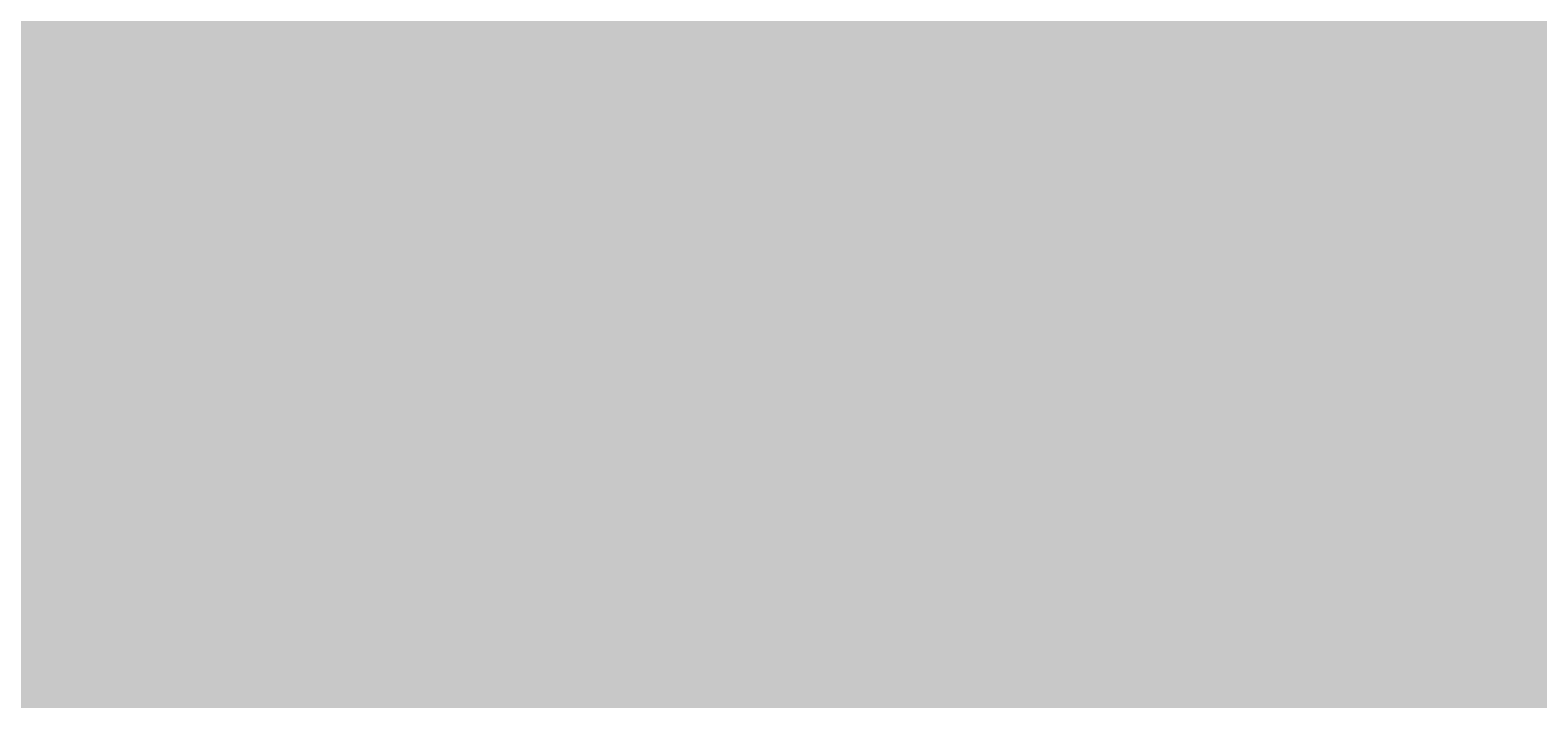
# Model space of a CAD drawing. Units: millimetres. Extents: x -22994 to 29398, y -19990 to 20176.
# Tile 108 of 135: x 237 to 296, y 98 to 124. Entities that reach past the tile are written whole.
import ezdxf

# ---------------------------------------------------------------- set-up
doc = ezdxf.new("R2010")
doc.units = ezdxf.units.MM
doc.header["$MEASUREMENT"] = 0
doc.layers.add('M-DIMS', color=2, linetype='Continuous', lineweight=18)
doc.styles.get("Standard").update_dxf_attribs({"font": 'arial.ttf'})
doc.dimstyles.get("Standard").update_dxf_attribs({"dimtxt": 0.18, "dimasz": 10000, "dimexe": 0.18, "dimexo": 0.0625, "dimgap": 0.09, "dimtad": 0, "dimtih": 1, "dimtoh": 1, "dimdec": 0, "dimzin": 0, "dimdsep": 46, "dimtxsty": 'Standard', "dimcen": 0.09, "dimadec": 0, "dimazin": 0, "dimtfac": 1, "dimtdec": 0, "dimtofl": 0, "dimtmove": 0, "dimatfit": 3, "dimfxl": 1, "dimtolj": 1, "dimtzin": 0, "dimlwd": 30, "dimarcsym": 0})

# ---------------------------------------------------------------- blocks, each defined once
blk = doc.blocks.new('*D2')
at = {"layer": 'Defpoints', "color": 0, "transparency": 16777216}
for p in [(6.677, 10.271), (290.852, 10.271), (290.852, -5.079)]:
    blk.add_point(p, dxfattribs=at)
at = {"layer": 'M-DIMS', "color": 0, "lineweight": -2, "transparency": 16777216}
for p, q in [((6.677, 10.209), (6.677, -5.259)), ((290.852, 10.209), (290.852, -5.259))]:
    blk.add_line(p, q, dxfattribs=at)
at = {"layer": 'M-DIMS', "color": 0, "lineweight": 30, "transparency": 16777216}
for p, q in [((-9993.323, -5.079), (-19993.323, -5.079)), ((10290.852, -5.079), (20290.852, -5.079))]:
    blk.add_line(p, q, dxfattribs=at)
at = {"layer": 'M-DIMS', "color": 0, "transparency": 16777216}
for points in [[(-9993.323, 1661.588), (-9993.323, -1671.745), (6.677, -5.079)], [(10290.852, 1661.588), (10290.852, -1671.745), (290.852, -5.079)]]:
    blk.add_solid(points, dxfattribs=at)
at = {"layer": 'M-DIMS', "color": 0, "transparency": 16777216, "insert": (148.765, -5.079), "char_height": 0.18, "attachment_point": 5}
blk.add_mtext('\\A1;284.2', dxfattribs=at)
blk = doc.blocks.new('*D3')
at = {"layer": 'Defpoints', "color": 0, "transparency": 16777216}
for p in [(110.265, 204.165), (110.265, 176.366), (95.833, 127.967)]:
    blk.add_point(p, dxfattribs=at)
at = {"layer": 'M-DIMS', "color": 0, "lineweight": -2, "transparency": 16777216}
for p, q in [((95.833, 128.03), (95.833, 204.345)), ((110.265, 176.429), (110.265, 204.345))]:
    blk.add_line(p, q, dxfattribs=at)
at = {"layer": 'M-DIMS', "color": 0, "lineweight": 30, "transparency": 16777216}
for p, q in [((-9904.167, 204.165), (-19904.167, 204.165)), ((10110.265, 204.165), (20110.265, 204.165))]:
    blk.add_line(p, q, dxfattribs=at)
at = {"layer": 'M-DIMS', "color": 0, "transparency": 16777216}
for points in [[(-9904.167, 1870.832), (-9904.167, -1462.501), (95.833, 204.165)], [(10110.265, 1870.832), (10110.265, -1462.501), (110.265, 204.165)]]:
    blk.add_solid(points, dxfattribs=at)
at = {"layer": 'M-DIMS', "color": 0, "transparency": 16777216, "insert": (103.049, 204.165), "char_height": 0.18, "attachment_point": 5}
blk.add_mtext('\\A1;14.432', dxfattribs=at)
blk = doc.blocks.new('*D4')
at = {"layer": 'Defpoints', "color": 0, "transparency": 16777216}
for p in [(116.265, 204.165), (110.265, 176.366), (116.265, 176.366)]:
    blk.add_point(p, dxfattribs=at)
at = {"layer": 'M-DIMS', "color": 0, "lineweight": -2, "transparency": 16777216}
for p, q in [((110.265, 176.429), (110.265, 204.345)), ((116.265, 176.429), (116.265, 204.345))]:
    blk.add_line(p, q, dxfattribs=at)
at = {"layer": 'M-DIMS', "color": 0, "lineweight": 30, "transparency": 16777216}
for p, q in [((-9889.735, 204.165), (-19889.735, 204.165)), ((10116.265, 204.165), (20116.265, 204.165))]:
    blk.add_line(p, q, dxfattribs=at)
at = {"layer": 'M-DIMS', "color": 0, "transparency": 16777216}
for points in [[(-9889.735, 1870.832), (-9889.735, -1462.501), (110.265, 204.165)], [(10116.265, 1870.832), (10116.265, -1462.501), (116.265, 204.165)]]:
    blk.add_solid(points, dxfattribs=at)
at = {"layer": 'M-DIMS', "color": 0, "transparency": 16777216, "insert": (113.265, 204.165), "char_height": 0.18, "attachment_point": 5}
blk.add_mtext('\\A1;6', dxfattribs=at)
blk = doc.blocks.new('*D5')
at = {"layer": 'Defpoints', "color": 0, "transparency": 16777216}
for p in [(181.265, 204.165), (116.265, 176.366), (181.265, 176.366)]:
    blk.add_point(p, dxfattribs=at)
at = {"layer": 'M-DIMS', "color": 0, "lineweight": -2, "transparency": 16777216}
for p, q in [((116.265, 176.429), (116.265, 204.345)), ((181.265, 176.429), (181.265, 204.345))]:
    blk.add_line(p, q, dxfattribs=at)
at = {"layer": 'M-DIMS', "color": 0, "lineweight": 30, "transparency": 16777216}
for p, q in [((-9883.735, 204.165), (-19883.735, 204.165)), ((10181.265, 204.165), (20181.265, 204.165))]:
    blk.add_line(p, q, dxfattribs=at)
at = {"layer": 'M-DIMS', "color": 0, "transparency": 16777216}
for points in [[(-9883.735, 1870.832), (-9883.735, -1462.501), (116.265, 204.165)], [(10181.265, 1870.832), (10181.265, -1462.501), (181.265, 204.165)]]:
    blk.add_solid(points, dxfattribs=at)
at = {"layer": 'M-DIMS', "color": 0, "transparency": 16777216, "insert": (148.765, 204.165), "char_height": 0.18, "attachment_point": 5}
blk.add_mtext('\\A1;65', dxfattribs=at)
blk = doc.blocks.new('*D6')
at = {"layer": 'Defpoints', "color": 0, "transparency": 16777216}
for p in [(187.265, 204.165), (181.265, 176.366), (187.265, 176.366)]:
    blk.add_point(p, dxfattribs=at)
at = {"layer": 'M-DIMS', "color": 0, "lineweight": -2, "transparency": 16777216}
for p, q in [((181.265, 176.429), (181.265, 204.345)), ((187.265, 176.429), (187.265, 204.345))]:
    blk.add_line(p, q, dxfattribs=at)
at = {"layer": 'M-DIMS', "color": 0, "lineweight": 30, "transparency": 16777216}
for p, q in [((-9818.735, 204.165), (-19818.735, 204.165)), ((10187.265, 204.165), (20187.265, 204.165))]:
    blk.add_line(p, q, dxfattribs=at)
at = {"layer": 'M-DIMS', "color": 0, "transparency": 16777216}
for points in [[(-9818.735, 1870.832), (-9818.735, -1462.501), (181.265, 204.165)], [(10187.265, 1870.832), (10187.265, -1462.501), (187.265, 204.165)]]:
    blk.add_solid(points, dxfattribs=at)
at = {"layer": 'M-DIMS', "color": 0, "transparency": 16777216, "insert": (184.265, 204.165), "char_height": 0.18, "attachment_point": 5}
blk.add_mtext('\\A1;6', dxfattribs=at)
blk = doc.blocks.new('*D7')
at = {"layer": 'Defpoints', "color": 0, "transparency": 16777216}
for p in [(201.697, 204.165), (187.265, 176.366), (201.697, 127.967)]:
    blk.add_point(p, dxfattribs=at)
at = {"layer": 'M-DIMS', "color": 0, "lineweight": -2, "transparency": 16777216}
for p, q in [((187.265, 176.429), (187.265, 204.345)), ((201.697, 128.03), (201.697, 204.345))]:
    blk.add_line(p, q, dxfattribs=at)
at = {"layer": 'M-DIMS', "color": 0, "lineweight": 30, "transparency": 16777216}
for p, q in [((-9812.735, 204.165), (-19812.735, 204.165)), ((10201.697, 204.165), (20201.697, 204.165))]:
    blk.add_line(p, q, dxfattribs=at)
at = {"layer": 'M-DIMS', "color": 0, "transparency": 16777216}
for points in [[(-9812.735, 1870.832), (-9812.735, -1462.501), (187.265, 204.165)], [(10201.697, 1870.832), (10201.697, -1462.501), (201.697, 204.165)]]:
    blk.add_solid(points, dxfattribs=at)
at = {"layer": 'M-DIMS', "color": 0, "transparency": 16777216, "insert": (194.481, 204.165), "char_height": 0.18, "attachment_point": 5}
blk.add_mtext('\\A1;14.432', dxfattribs=at)
blk = doc.blocks.new('*D8')
at = {"layer": 'Defpoints', "color": 0, "transparency": 16777216}
for p in [(227.648, 204.165), (227.648, 146.73), (201.697, 127.967)]:
    blk.add_point(p, dxfattribs=at)
at = {"layer": 'M-DIMS', "color": 0, "lineweight": -2, "transparency": 16777216}
for p, q in [((201.697, 128.03), (201.697, 204.345)), ((227.648, 146.792), (227.648, 204.345))]:
    blk.add_line(p, q, dxfattribs=at)
at = {"layer": 'M-DIMS', "color": 0, "lineweight": 30, "transparency": 16777216}
for p, q in [((-9798.303, 204.165), (-19798.303, 204.165)), ((10227.648, 204.165), (20227.648, 204.165))]:
    blk.add_line(p, q, dxfattribs=at)
at = {"layer": 'M-DIMS', "color": 0, "transparency": 16777216}
for points in [[(-9798.303, 1870.832), (-9798.303, -1462.501), (201.697, 204.165)], [(10227.648, 1870.832), (10227.648, -1462.501), (227.648, 204.165)]]:
    blk.add_solid(points, dxfattribs=at)
at = {"layer": 'M-DIMS', "color": 0, "transparency": 16777216, "insert": (214.673, 204.165), "char_height": 0.18, "attachment_point": 5}
blk.add_mtext('\\A1;25.95', dxfattribs=at)
blk = doc.blocks.new('*D9')
at = {"layer": 'Defpoints', "color": 0, "transparency": 16777216}
for p in [(187.265, 176.366), (306.202, 176.366), (290.852, 10.271)]:
    blk.add_point(p, dxfattribs=at)
at = {"layer": 'M-DIMS', "color": 0, "lineweight": 30, "transparency": 16777216}
for p, q in [((306.202, 10176.366), (306.202, 20176.366)), ((306.202, -9989.729), (306.202, -19989.729))]:
    blk.add_line(p, q, dxfattribs=at)
at = {"layer": 'M-DIMS', "color": 0, "lineweight": -2, "transparency": 16777216}
for p, q in [((187.327, 176.366), (306.382, 176.366)), ((290.915, 10.271), (306.382, 10.271))]:
    blk.add_line(p, q, dxfattribs=at)
at = {"layer": 'M-DIMS', "color": 0, "transparency": 16777216}
for points in [[(-1360.465, 10176.366), (1972.869, 10176.366), (306.202, 176.366)], [(-1360.465, -9989.729), (1972.869, -9989.729), (306.202, 10.271)]]:
    blk.add_solid(points, dxfattribs=at)
at = {"layer": 'M-DIMS', "color": 0, "transparency": 16777216, "insert": (306.202, 93.319), "char_height": 0.18, "attachment_point": 5}
blk.add_mtext('\\A1;166.1', dxfattribs=at)
blk = doc.blocks.new('*D10')
at = {"layer": 'Defpoints', "color": 0, "transparency": 16777216}
for p in [(125.65, 136.071), (133.346, 136.071), (133.346, -5.079)]:
    blk.add_point(p, dxfattribs=at)
at = {"layer": 'M-DIMS', "color": 0, "lineweight": -2, "transparency": 16777216}
for p, q in [((125.65, 136.009), (125.65, -5.259)), ((133.346, 136.009), (133.346, -5.259))]:
    blk.add_line(p, q, dxfattribs=at)
at = {"layer": 'M-DIMS', "color": 0, "lineweight": 30, "transparency": 16777216}
for p, q in [((-9874.35, -5.079), (-19874.35, -5.079)), ((10133.346, -5.079), (20133.346, -5.079))]:
    blk.add_line(p, q, dxfattribs=at)
at = {"layer": 'M-DIMS', "color": 0, "transparency": 16777216}
for points in [[(-9874.35, 1661.588), (-9874.35, -1671.745), (125.65, -5.079)], [(10133.346, 1661.588), (10133.346, -1671.745), (133.346, -5.079)]]:
    blk.add_solid(points, dxfattribs=at)
at = {"layer": 'M-DIMS', "color": 0, "transparency": 16777216, "insert": (129.498, -5.079), "char_height": 0.18, "attachment_point": 5}
blk.add_mtext('\\A1;7.696', dxfattribs=at)
blk = doc.blocks.new('*D11')
at = {"layer": 'Defpoints', "color": 0, "transparency": 16777216}
for p in [(133.346, 136.071), (135.65, 136.071), (135.65, -5.079)]:
    blk.add_point(p, dxfattribs=at)
at = {"layer": 'M-DIMS', "color": 0, "lineweight": -2, "transparency": 16777216}
for p, q in [((133.346, 136.009), (133.346, -5.259)), ((135.65, 136.009), (135.65, -5.259))]:
    blk.add_line(p, q, dxfattribs=at)
at = {"layer": 'M-DIMS', "color": 0, "lineweight": 30, "transparency": 16777216}
for p, q in [((-9866.654, -5.079), (-19866.654, -5.079)), ((10135.65, -5.079), (20135.65, -5.079))]:
    blk.add_line(p, q, dxfattribs=at)
at = {"layer": 'M-DIMS', "color": 0, "transparency": 16777216}
for points in [[(-9866.654, 1661.588), (-9866.654, -1671.745), (133.346, -5.079)], [(10135.65, 1661.588), (10135.65, -1671.745), (135.65, -5.079)]]:
    blk.add_solid(points, dxfattribs=at)
at = {"layer": 'M-DIMS', "color": 0, "transparency": 16777216, "insert": (134.498, -5.079), "char_height": 0.18, "attachment_point": 5}
blk.add_mtext('\\A1;2.304', dxfattribs=at)
blk = doc.blocks.new('*D12')
at = {"layer": 'Defpoints', "color": 0, "transparency": 16777216}
for p in [(135.65, 136.071), (145.65, 136.071), (145.65, -5.079)]:
    blk.add_point(p, dxfattribs=at)
at = {"layer": 'M-DIMS', "color": 0, "lineweight": -2, "transparency": 16777216}
for p, q in [((135.65, 136.009), (135.65, -5.259)), ((145.65, 136.009), (145.65, -5.259))]:
    blk.add_line(p, q, dxfattribs=at)
at = {"layer": 'M-DIMS', "color": 0, "lineweight": 30, "transparency": 16777216}
for p, q in [((-9864.35, -5.079), (-19864.35, -5.079)), ((10145.65, -5.079), (20145.65, -5.079))]:
    blk.add_line(p, q, dxfattribs=at)
at = {"layer": 'M-DIMS', "color": 0, "transparency": 16777216}
for points in [[(-9864.35, 1661.588), (-9864.35, -1671.745), (135.65, -5.079)], [(10145.65, 1661.588), (10145.65, -1671.745), (145.65, -5.079)]]:
    blk.add_solid(points, dxfattribs=at)
at = {"layer": 'M-DIMS', "color": 0, "transparency": 16777216, "insert": (140.65, -5.079), "char_height": 0.18, "attachment_point": 5}
blk.add_mtext('\\A1;10', dxfattribs=at)
blk = doc.blocks.new('*D13')
at = {"layer": 'Defpoints', "color": 0, "transparency": 16777216}
for p in [(145.65, 136.071), (155.65, 136.071), (155.65, -5.079)]:
    blk.add_point(p, dxfattribs=at)
at = {"layer": 'M-DIMS', "color": 0, "lineweight": -2, "transparency": 16777216}
for p, q in [((145.65, 136.009), (145.65, -5.259)), ((155.65, 136.009), (155.65, -5.259))]:
    blk.add_line(p, q, dxfattribs=at)
at = {"layer": 'M-DIMS', "color": 0, "lineweight": 30, "transparency": 16777216}
for p, q in [((-9854.35, -5.079), (-19854.35, -5.079)), ((10155.65, -5.079), (20155.65, -5.079))]:
    blk.add_line(p, q, dxfattribs=at)
at = {"layer": 'M-DIMS', "color": 0, "transparency": 16777216}
for points in [[(-9854.35, 1661.588), (-9854.35, -1671.745), (145.65, -5.079)], [(10155.65, 1661.588), (10155.65, -1671.745), (155.65, -5.079)]]:
    blk.add_solid(points, dxfattribs=at)
at = {"layer": 'M-DIMS', "color": 0, "transparency": 16777216, "insert": (150.65, -5.079), "char_height": 0.18, "attachment_point": 5}
blk.add_mtext('\\A1;10', dxfattribs=at)
blk = doc.blocks.new('*D14')
at = {"layer": 'Defpoints', "color": 0, "transparency": 16777216}
for p in [(155.65, 136.071), (165.65, 136.071), (165.65, -5.079)]:
    blk.add_point(p, dxfattribs=at)
at = {"layer": 'M-DIMS', "color": 0, "lineweight": -2, "transparency": 16777216}
for p, q in [((155.65, 136.009), (155.65, -5.259)), ((165.65, 136.009), (165.65, -5.259))]:
    blk.add_line(p, q, dxfattribs=at)
at = {"layer": 'M-DIMS', "color": 0, "lineweight": 30, "transparency": 16777216}
for p, q in [((-9844.35, -5.079), (-19844.35, -5.079)), ((10165.65, -5.079), (20165.65, -5.079))]:
    blk.add_line(p, q, dxfattribs=at)
at = {"layer": 'M-DIMS', "color": 0, "transparency": 16777216}
for points in [[(-9844.35, 1661.588), (-9844.35, -1671.745), (155.65, -5.079)], [(10165.65, 1661.588), (10165.65, -1671.745), (165.65, -5.079)]]:
    blk.add_solid(points, dxfattribs=at)
at = {"layer": 'M-DIMS', "color": 0, "transparency": 16777216, "insert": (160.65, -5.079), "char_height": 0.18, "attachment_point": 5}
blk.add_mtext('\\A1;10', dxfattribs=at)
blk = doc.blocks.new('*D15')
at = {"layer": 'Defpoints', "color": 0, "transparency": 16777216}
for p in [(173.346, 154.788), (173.346, 136.071), (306.202, 136.071)]:
    blk.add_point(p, dxfattribs=at)
at = {"layer": 'M-DIMS', "color": 0, "lineweight": 30, "transparency": 16777216}
for p, q in [((306.202, 10154.788), (306.202, 20154.788)), ((306.202, -9863.929), (306.202, -19863.929))]:
    blk.add_line(p, q, dxfattribs=at)
at = {"layer": 'M-DIMS', "color": 0, "lineweight": -2, "transparency": 16777216}
for p, q in [((173.408, 154.788), (306.382, 154.788)), ((173.408, 136.071), (306.382, 136.071))]:
    blk.add_line(p, q, dxfattribs=at)
at = {"layer": 'M-DIMS', "color": 0, "transparency": 16777216}
for points in [[(-1360.465, 10154.788), (1972.869, 10154.788), (306.202, 154.788)], [(-1360.465, -9863.929), (1972.869, -9863.929), (306.202, 136.071)]]:
    blk.add_solid(points, dxfattribs=at)
at = {"layer": 'M-DIMS', "color": 0, "transparency": 16777216, "insert": (306.202, 145.43), "char_height": 0.18, "attachment_point": 5}
blk.add_mtext('\\A1;18.717', dxfattribs=at)
blk = doc.blocks.new('*D16')
at = {"layer": 'Defpoints', "color": 0, "transparency": 16777216}
for p in [(120.17, 204.165), (110.466, 48.035), (120.17, 48.035)]:
    blk.add_point(p, dxfattribs=at)
at = {"layer": 'M-DIMS', "color": 0, "lineweight": -2, "transparency": 16777216}
for p, q in [((110.466, 48.097), (110.466, 204.345)), ((120.17, 48.097), (120.17, 204.345))]:
    blk.add_line(p, q, dxfattribs=at)
at = {"layer": 'M-DIMS', "color": 0, "lineweight": 30, "transparency": 16777216}
for p, q in [((-9889.534, 204.165), (-19889.534, 204.165)), ((10120.17, 204.165), (20120.17, 204.165))]:
    blk.add_line(p, q, dxfattribs=at)
at = {"layer": 'M-DIMS', "color": 0, "transparency": 16777216}
for points in [[(-9889.534, 1870.832), (-9889.534, -1462.501), (110.466, 204.165)], [(10120.17, 1870.832), (10120.17, -1462.501), (120.17, 204.165)]]:
    blk.add_solid(points, dxfattribs=at)
at = {"layer": 'M-DIMS', "color": 0, "transparency": 16777216, "insert": (115.318, 204.165), "char_height": 0.18, "attachment_point": 5}
blk.add_mtext('\\A1;9.704', dxfattribs=at)
blk = doc.blocks.new('*D17')
at = {"layer": 'Defpoints', "color": 0, "transparency": 16777216}
for p in [(126.17, 204.165), (120.17, 48.035), (126.17, 48.035)]:
    blk.add_point(p, dxfattribs=at)
at = {"layer": 'M-DIMS', "color": 0, "lineweight": -2, "transparency": 16777216}
for p, q in [((120.17, 48.097), (120.17, 204.345)), ((126.17, 48.097), (126.17, 204.345))]:
    blk.add_line(p, q, dxfattribs=at)
at = {"layer": 'M-DIMS', "color": 0, "lineweight": 30, "transparency": 16777216}
for p, q in [((-9879.83, 204.165), (-19879.83, 204.165)), ((10126.17, 204.165), (20126.17, 204.165))]:
    blk.add_line(p, q, dxfattribs=at)
at = {"layer": 'M-DIMS', "color": 0, "transparency": 16777216}
for points in [[(-9879.83, 1870.832), (-9879.83, -1462.501), (120.17, 204.165)], [(10126.17, 1870.832), (10126.17, -1462.501), (126.17, 204.165)]]:
    blk.add_solid(points, dxfattribs=at)
at = {"layer": 'M-DIMS', "color": 0, "transparency": 16777216, "insert": (123.17, 204.165), "char_height": 0.18, "attachment_point": 5}
blk.add_mtext('\\A1;6', dxfattribs=at)
blk = doc.blocks.new('*D18')
at = {"layer": 'Defpoints', "color": 0, "transparency": 16777216}
for p in [(132.17, 204.165), (126.17, 48.035), (132.17, 48.035)]:
    blk.add_point(p, dxfattribs=at)
at = {"layer": 'M-DIMS', "color": 0, "lineweight": -2, "transparency": 16777216}
for p, q in [((126.17, 48.097), (126.17, 204.345)), ((132.17, 48.097), (132.17, 204.345))]:
    blk.add_line(p, q, dxfattribs=at)
at = {"layer": 'M-DIMS', "color": 0, "lineweight": 30, "transparency": 16777216}
for p, q in [((-9873.83, 204.165), (-19873.83, 204.165)), ((10132.17, 204.165), (20132.17, 204.165))]:
    blk.add_line(p, q, dxfattribs=at)
at = {"layer": 'M-DIMS', "color": 0, "transparency": 16777216}
for points in [[(-9873.83, 1870.832), (-9873.83, -1462.501), (126.17, 204.165)], [(10132.17, 1870.832), (10132.17, -1462.501), (132.17, 204.165)]]:
    blk.add_solid(points, dxfattribs=at)
at = {"layer": 'M-DIMS', "color": 0, "transparency": 16777216, "insert": (129.17, 204.165), "char_height": 0.18, "attachment_point": 5}
blk.add_mtext('\\A1;6', dxfattribs=at)
blk = doc.blocks.new('*D19')
at = {"layer": 'Defpoints', "color": 0, "transparency": 16777216}
for p in [(138.17, 204.165), (132.17, 48.035), (138.17, 48.035)]:
    blk.add_point(p, dxfattribs=at)
at = {"layer": 'M-DIMS', "color": 0, "lineweight": -2, "transparency": 16777216}
for p, q in [((132.17, 48.097), (132.17, 204.345)), ((138.17, 48.097), (138.17, 204.345))]:
    blk.add_line(p, q, dxfattribs=at)
at = {"layer": 'M-DIMS', "color": 0, "lineweight": 30, "transparency": 16777216}
for p, q in [((-9867.83, 204.165), (-19867.83, 204.165)), ((10138.17, 204.165), (20138.17, 204.165))]:
    blk.add_line(p, q, dxfattribs=at)
at = {"layer": 'M-DIMS', "color": 0, "transparency": 16777216}
for points in [[(-9867.83, 1870.832), (-9867.83, -1462.501), (132.17, 204.165)], [(10138.17, 1870.832), (10138.17, -1462.501), (138.17, 204.165)]]:
    blk.add_solid(points, dxfattribs=at)
at = {"layer": 'M-DIMS', "color": 0, "transparency": 16777216, "insert": (135.17, 204.165), "char_height": 0.18, "attachment_point": 5}
blk.add_mtext('\\A1;6', dxfattribs=at)
blk = doc.blocks.new('*D20')
at = {"layer": 'Defpoints', "color": 0, "transparency": 16777216}
for p in [(144.17, 204.165), (138.17, 48.035), (144.17, 48.035)]:
    blk.add_point(p, dxfattribs=at)
at = {"layer": 'M-DIMS', "color": 0, "lineweight": -2, "transparency": 16777216}
for p, q in [((138.17, 48.097), (138.17, 204.345)), ((144.17, 48.097), (144.17, 204.345))]:
    blk.add_line(p, q, dxfattribs=at)
at = {"layer": 'M-DIMS', "color": 0, "lineweight": 30, "transparency": 16777216}
for p, q in [((-9861.83, 204.165), (-19861.83, 204.165)), ((10144.17, 204.165), (20144.17, 204.165))]:
    blk.add_line(p, q, dxfattribs=at)
at = {"layer": 'M-DIMS', "color": 0, "transparency": 16777216}
for points in [[(-9861.83, 1870.832), (-9861.83, -1462.501), (138.17, 204.165)], [(10144.17, 1870.832), (10144.17, -1462.501), (144.17, 204.165)]]:
    blk.add_solid(points, dxfattribs=at)
at = {"layer": 'M-DIMS', "color": 0, "transparency": 16777216, "insert": (141.17, 204.165), "char_height": 0.18, "attachment_point": 5}
blk.add_mtext('\\A1;6', dxfattribs=at)
blk = doc.blocks.new('*D21')
at = {"layer": 'Defpoints', "color": 0, "transparency": 16777216}
for p in [(149.116, 204.165), (144.17, 48.035), (149.116, 48.035)]:
    blk.add_point(p, dxfattribs=at)
at = {"layer": 'M-DIMS', "color": 0, "lineweight": -2, "transparency": 16777216}
for p, q in [((144.17, 48.097), (144.17, 204.345)), ((149.116, 48.097), (149.116, 204.345))]:
    blk.add_line(p, q, dxfattribs=at)
at = {"layer": 'M-DIMS', "color": 0, "lineweight": 30, "transparency": 16777216}
for p, q in [((-9855.83, 204.165), (-19855.83, 204.165)), ((10149.116, 204.165), (20149.116, 204.165))]:
    blk.add_line(p, q, dxfattribs=at)
at = {"layer": 'M-DIMS', "color": 0, "transparency": 16777216}
for points in [[(-9855.83, 1870.832), (-9855.83, -1462.501), (144.17, 204.165)], [(10149.116, 1870.832), (10149.116, -1462.501), (149.116, 204.165)]]:
    blk.add_solid(points, dxfattribs=at)
at = {"layer": 'M-DIMS', "color": 0, "transparency": 16777216, "insert": (146.643, 204.165), "char_height": 0.18, "attachment_point": 5}
blk.add_mtext('\\A1;4.945', dxfattribs=at)
blk = doc.blocks.new('*D22')
at = {"layer": 'Defpoints', "color": 0, "transparency": 16777216}
for p in [(149.116, 30.99), (155.116, 30.99), (155.116, -5.079)]:
    blk.add_point(p, dxfattribs=at)
at = {"layer": 'M-DIMS', "color": 0, "lineweight": -2, "transparency": 16777216}
for p, q in [((149.116, 30.927), (149.116, -5.259)), ((155.116, 30.927), (155.116, -5.259))]:
    blk.add_line(p, q, dxfattribs=at)
at = {"layer": 'M-DIMS', "color": 0, "lineweight": 30, "transparency": 16777216}
for p, q in [((-9850.884, -5.079), (-19850.884, -5.079)), ((10155.116, -5.079), (20155.116, -5.079))]:
    blk.add_line(p, q, dxfattribs=at)
at = {"layer": 'M-DIMS', "color": 0, "transparency": 16777216}
for points in [[(-9850.884, 1661.588), (-9850.884, -1671.745), (149.116, -5.079)], [(10155.116, 1661.588), (10155.116, -1671.745), (155.116, -5.079)]]:
    blk.add_solid(points, dxfattribs=at)
at = {"layer": 'M-DIMS', "color": 0, "transparency": 16777216, "insert": (152.116, -5.079), "char_height": 0.18, "attachment_point": 5}
blk.add_mtext('\\A1;6', dxfattribs=at)
blk = doc.blocks.new('*D23')
at = {"layer": 'Defpoints', "color": 0, "transparency": 16777216}
for p in [(155.116, 30.99), (161.116, 30.99), (161.116, -5.079)]:
    blk.add_point(p, dxfattribs=at)
at = {"layer": 'M-DIMS', "color": 0, "lineweight": -2, "transparency": 16777216}
for p, q in [((155.116, 30.927), (155.116, -5.259)), ((161.116, 30.927), (161.116, -5.259))]:
    blk.add_line(p, q, dxfattribs=at)
at = {"layer": 'M-DIMS', "color": 0, "lineweight": 30, "transparency": 16777216}
for p, q in [((-9844.884, -5.079), (-19844.884, -5.079)), ((10161.116, -5.079), (20161.116, -5.079))]:
    blk.add_line(p, q, dxfattribs=at)
at = {"layer": 'M-DIMS', "color": 0, "transparency": 16777216}
for points in [[(-9844.884, 1661.588), (-9844.884, -1671.745), (155.116, -5.079)], [(10161.116, 1661.588), (10161.116, -1671.745), (161.116, -5.079)]]:
    blk.add_solid(points, dxfattribs=at)
at = {"layer": 'M-DIMS', "color": 0, "transparency": 16777216, "insert": (158.116, -5.079), "char_height": 0.18, "attachment_point": 5}
blk.add_mtext('\\A1;6', dxfattribs=at)
blk = doc.blocks.new('*D24')
at = {"layer": 'Defpoints', "color": 0, "transparency": 16777216}
for p in [(161.116, 30.99), (166.439, 30.99), (166.439, -5.079)]:
    blk.add_point(p, dxfattribs=at)
at = {"layer": 'M-DIMS', "color": 0, "lineweight": -2, "transparency": 16777216}
for p, q in [((161.116, 30.927), (161.116, -5.259)), ((166.439, 30.927), (166.439, -5.259))]:
    blk.add_line(p, q, dxfattribs=at)
at = {"layer": 'M-DIMS', "color": 0, "lineweight": 30, "transparency": 16777216}
for p, q in [((-9838.884, -5.079), (-19838.884, -5.079)), ((10166.439, -5.079), (20166.439, -5.079))]:
    blk.add_line(p, q, dxfattribs=at)
at = {"layer": 'M-DIMS', "color": 0, "transparency": 16777216}
for points in [[(-9838.884, 1661.588), (-9838.884, -1671.745), (161.116, -5.079)], [(10166.439, 1661.588), (10166.439, -1671.745), (166.439, -5.079)]]:
    blk.add_solid(points, dxfattribs=at)
at = {"layer": 'M-DIMS', "color": 0, "transparency": 16777216, "insert": (163.777, -5.079), "char_height": 0.18, "attachment_point": 5}
blk.add_mtext('\\A1;5.323', dxfattribs=at)
blk = doc.blocks.new('*D25')
at = {"layer": 'Defpoints', "color": 0, "transparency": 16777216}
for p in [(166.439, 30.99), (172.439, 30.99), (172.439, -5.079)]:
    blk.add_point(p, dxfattribs=at)
at = {"layer": 'M-DIMS', "color": 0, "lineweight": -2, "transparency": 16777216}
for p, q in [((166.439, 30.927), (166.439, -5.259)), ((172.439, 30.927), (172.439, -5.259))]:
    blk.add_line(p, q, dxfattribs=at)
at = {"layer": 'M-DIMS', "color": 0, "lineweight": 30, "transparency": 16777216}
for p, q in [((-9833.561, -5.079), (-19833.561, -5.079)), ((10172.439, -5.079), (20172.439, -5.079))]:
    blk.add_line(p, q, dxfattribs=at)
at = {"layer": 'M-DIMS', "color": 0, "transparency": 16777216}
for points in [[(-9833.561, 1661.588), (-9833.561, -1671.745), (166.439, -5.079)], [(10172.439, 1661.588), (10172.439, -1671.745), (172.439, -5.079)]]:
    blk.add_solid(points, dxfattribs=at)
at = {"layer": 'M-DIMS', "color": 0, "transparency": 16777216, "insert": (169.439, -5.079), "char_height": 0.18, "attachment_point": 5}
blk.add_mtext('\\A1;6', dxfattribs=at)
blk = doc.blocks.new('*D26')
at = {"layer": 'Defpoints', "color": 0, "transparency": 16777216}
for p in [(172.439, 30.99), (178.439, 30.99), (178.439, -5.079)]:
    blk.add_point(p, dxfattribs=at)
at = {"layer": 'M-DIMS', "color": 0, "lineweight": -2, "transparency": 16777216}
for p, q in [((172.439, 30.927), (172.439, -5.259)), ((178.439, 30.927), (178.439, -5.259))]:
    blk.add_line(p, q, dxfattribs=at)
at = {"layer": 'M-DIMS', "color": 0, "lineweight": 30, "transparency": 16777216}
for p, q in [((-9827.561, -5.079), (-19827.561, -5.079)), ((10178.439, -5.079), (20178.439, -5.079))]:
    blk.add_line(p, q, dxfattribs=at)
at = {"layer": 'M-DIMS', "color": 0, "transparency": 16777216}
for points in [[(-9827.561, 1661.588), (-9827.561, -1671.745), (172.439, -5.079)], [(10178.439, 1661.588), (10178.439, -1671.745), (178.439, -5.079)]]:
    blk.add_solid(points, dxfattribs=at)
at = {"layer": 'M-DIMS', "color": 0, "transparency": 16777216, "insert": (175.439, -5.079), "char_height": 0.18, "attachment_point": 5}
blk.add_mtext('\\A1;6', dxfattribs=at)
blk = doc.blocks.new('*D27')
at = {"layer": 'Defpoints', "color": 0, "transparency": 16777216}
for p in [(178.439, 30.99), (188.117, 30.99), (188.117, -5.079)]:
    blk.add_point(p, dxfattribs=at)
at = {"layer": 'M-DIMS', "color": 0, "lineweight": -2, "transparency": 16777216}
for p, q in [((178.439, 30.927), (178.439, -5.259)), ((188.117, 30.927), (188.117, -5.259))]:
    blk.add_line(p, q, dxfattribs=at)
at = {"layer": 'M-DIMS', "color": 0, "lineweight": 30, "transparency": 16777216}
for p, q in [((-9821.561, -5.079), (-19821.561, -5.079)), ((10188.117, -5.079), (20188.117, -5.079))]:
    blk.add_line(p, q, dxfattribs=at)
at = {"layer": 'M-DIMS', "color": 0, "transparency": 16777216}
for points in [[(-9821.561, 1661.588), (-9821.561, -1671.745), (178.439, -5.079)], [(10188.117, 1661.588), (10188.117, -1671.745), (188.117, -5.079)]]:
    blk.add_solid(points, dxfattribs=at)
at = {"layer": 'M-DIMS', "color": 0, "transparency": 16777216, "insert": (183.278, -5.079), "char_height": 0.18, "attachment_point": 5}
blk.add_mtext('\\A1;9.679', dxfattribs=at)
blk = doc.blocks.new('*D28')
at = {"layer": 'Defpoints', "color": 0, "transparency": 16777216}
for p in [(188.117, 48.035), (306.202, 48.035), (188.117, 30.99)]:
    blk.add_point(p, dxfattribs=at)
at = {"layer": 'M-DIMS', "color": 0, "lineweight": 30, "transparency": 16777216}
for p, q in [((306.202, 10048.035), (306.202, 20048.035)), ((306.202, -9969.01), (306.202, -19969.01))]:
    blk.add_line(p, q, dxfattribs=at)
at = {"layer": 'M-DIMS', "color": 0, "lineweight": -2, "transparency": 16777216}
for p, q in [((188.18, 48.035), (306.382, 48.035)), ((188.18, 30.99), (306.382, 30.99))]:
    blk.add_line(p, q, dxfattribs=at)
at = {"layer": 'M-DIMS', "color": 0, "transparency": 16777216}
for points in [[(-1360.465, 10048.035), (1972.869, 10048.035), (306.202, 48.035)], [(-1360.465, -9969.01), (1972.869, -9969.01), (306.202, 30.99)]]:
    blk.add_solid(points, dxfattribs=at)
at = {"layer": 'M-DIMS', "color": 0, "transparency": 16777216, "insert": (306.202, 39.512), "char_height": 0.18, "attachment_point": 5}
blk.add_mtext('\\A1;17.045', dxfattribs=at)
blk = doc.blocks.new('*D29')
at = {"layer": 'Defpoints', "color": 0, "transparency": 16777216}
for p in [(36.801, 80.045), (64.03, 80.045)]:
    blk.add_point(p, dxfattribs=at)
at = {"layer": 'M-DIMS', "color": 0, "lineweight": -2, "transparency": 16777216}
for p, q in [((50.415, 79.955), (50.415, 80.135)), ((50.325, 80.045), (50.505, 80.045))]:
    blk.add_line(p, q, dxfattribs=at)
at = {"layer": 'M-DIMS', "color": 0, "lineweight": 30, "transparency": 16777216}
blk.add_line((20064.03, 80.03), (10064.03, 80.038), dxfattribs=at)
at = {"layer": 'M-DIMS', "color": 0, "transparency": 16777216}
blk.add_solid([(10064.031, 1746.704), (10064.028, -1586.629), (64.03, 80.045)], dxfattribs=at)
at = {"layer": 'M-DIMS', "color": 0, "transparency": 16777216, "insert": (20064.521, 80.03), "char_height": 0.18, "attachment_point": 5}
blk.add_mtext('\\A1;∅27.23', dxfattribs=at)
blk = doc.blocks.new('*D30')
at = {"layer": 'Defpoints', "color": 0, "transparency": 16777216}
for p in [(216.315, 146.729), (238.982, 146.73)]:
    blk.add_point(p, dxfattribs=at)
at = {"layer": 'M-DIMS', "color": 0, "lineweight": 30, "transparency": 16777216}
blk.add_line((20238.982, 147.496), (10238.982, 147.113), dxfattribs=at)
at = {"layer": 'M-DIMS', "color": 0, "lineweight": -2, "transparency": 16777216}
for p, q in [((227.558, 146.73), (227.738, 146.73)), ((227.648, 146.64), (227.648, 146.82))]:
    blk.add_line(p, q, dxfattribs=at)
at = {"layer": 'M-DIMS', "color": 0, "transparency": 16777216}
blk.add_solid([(10238.918, 1813.78), (10239.046, -1519.554), (238.982, 146.73)], dxfattribs=at)
at = {"layer": 'M-DIMS', "color": 0, "transparency": 16777216, "insert": (20239.544, 147.496), "char_height": 0.18, "attachment_point": 5}
blk.add_mtext('\\A1;∅22.667', dxfattribs=at)
blk = doc.blocks.new('*D31')
at = {"layer": 'Defpoints', "color": 0, "transparency": 16777216}
for p in [(223.164, 146.729), (232.133, 146.73)]:
    blk.add_point(p, dxfattribs=at)
at = {"layer": 'M-DIMS', "color": 0, "lineweight": 30, "transparency": 16777216}
blk.add_line((20232.133, 148.666), (10232.133, 147.698), dxfattribs=at)
at = {"layer": 'M-DIMS', "color": 0, "lineweight": -2, "transparency": 16777216}
for p, q in [((227.558, 146.73), (227.738, 146.73)), ((227.648, 146.64), (227.648, 146.82))]:
    blk.add_line(p, q, dxfattribs=at)
at = {"layer": 'M-DIMS', "color": 0, "transparency": 16777216}
blk.add_solid([(10231.971, 1814.364), (10232.294, -1518.969), (232.133, 146.73)], dxfattribs=at)
at = {"layer": 'M-DIMS', "color": 0, "transparency": 16777216, "insert": (20232.625, 148.666), "char_height": 0.18, "attachment_point": 5}
blk.add_mtext('\\A1;∅8.969', dxfattribs=at)
blk = doc.blocks.new('*D33')
at = {"layer": 'Defpoints', "color": 0, "transparency": 16777216}
for p in [(229.561, 154.377), (232.997, 153.351)]:
    blk.add_point(p, dxfattribs=at)
at = {"layer": 'M-DIMS', "color": 0, "lineweight": -2, "transparency": 16777216}
for p, q in [((229.471, 154.377), (229.651, 154.377)), ((229.561, 154.287), (229.561, 154.467))]:
    blk.add_line(p, q, dxfattribs=at)
at = {"layer": 'M-DIMS', "color": 0, "lineweight": 30, "transparency": 16777216}
for p, q in [((19396.339, -5570.838), (9814.668, -2708.743)), ((29396.339, -5570.838), (19396.339, -5570.838))]:
    blk.add_line(p, q, dxfattribs=at)
at = {"layer": 'M-DIMS', "color": 0, "transparency": 16777216}
blk.add_solid([(10291.684, -1111.798), (9337.652, -4305.689), (232.997, 153.351)], dxfattribs=at)
at = {"layer": 'M-DIMS', "color": 0, "transparency": 16777216, "insert": (29397.012, -5570.838), "char_height": 0.18, "attachment_point": 5}
blk.add_mtext('\\A1;6X R3.586', dxfattribs=at)
blk = doc.blocks.new('*D34')
at = {"layer": 'Defpoints', "color": 0, "transparency": 16777216}
for p in [(178.58, 122.895), (176.812, 121.128)]:
    blk.add_point(p, dxfattribs=at)
at = {"layer": 'M-DIMS', "color": 0, "lineweight": 30, "transparency": 16777216}
for p, q in [((14322.436, 14263.311), (7250.508, 7193.103)), ((24322.436, 14263.311), (14322.436, 14263.311))]:
    blk.add_line(p, q, dxfattribs=at)
at = {"layer": 'M-DIMS', "color": 0, "lineweight": -2, "transparency": 16777216}
for p, q in [((176.722, 121.128), (176.902, 121.128)), ((176.812, 121.038), (176.812, 121.218))]:
    blk.add_line(p, q, dxfattribs=at)
at = {"layer": 'M-DIMS', "color": 0, "transparency": 16777216}
blk.add_solid([(6072.14, 8371.758), (8428.876, 6014.448), (178.58, 122.895)], dxfattribs=at)
at = {"layer": 'M-DIMS', "color": 0, "transparency": 16777216, "insert": (24322.97, 14263.311), "char_height": 0.18, "attachment_point": 5}
blk.add_mtext('\\A1;6X R2.5', dxfattribs=at)
blk = doc.blocks.new('*D36')
at = {"layer": 'Defpoints', "color": 0, "transparency": 16777216}
for p in [(46.39, 31.303), (46.387, 26.593)]:
    blk.add_point(p, dxfattribs=at)
at = {"layer": 'M-DIMS', "color": 0, "lineweight": 30, "transparency": 16777216}
for p, q in [((57.15, 20031.301), (51.77, 10031.302)), ((10057.15, 20031.301), (57.15, 20031.301))]:
    blk.add_line(p, q, dxfattribs=at)
at = {"layer": 'M-DIMS', "color": 0, "lineweight": -2, "transparency": 16777216}
for p, q in [((46.299, 28.948), (46.479, 28.948)), ((46.389, 28.858), (46.389, 29.038))]:
    blk.add_line(p, q, dxfattribs=at)
at = {"layer": 'M-DIMS', "color": 0, "transparency": 16777216}
blk.add_solid([(-1614.896, 10032.199), (1718.436, 10030.405), (46.39, 31.303)], dxfattribs=at)
at = {"layer": 'M-DIMS', "color": 0, "transparency": 16777216, "insert": (10057.554, 20031.301), "char_height": 0.18, "attachment_point": 5}
blk.add_mtext('\\A1;∅4.71', dxfattribs=at)
blk = doc.blocks.new('*D37')
at = {"layer": 'Defpoints', "color": 0, "transparency": 16777216}
for p in [(54.834, 118.615), (59.494, 118.614)]:
    blk.add_point(p, dxfattribs=at)
at = {"layer": 'M-DIMS', "color": 0, "lineweight": -2, "transparency": 16777216}
for p, q in [((57.074, 118.614), (57.254, 118.614)), ((57.164, 118.524), (57.164, 118.704))]:
    blk.add_line(p, q, dxfattribs=at)
at = {"layer": 'M-DIMS', "color": 0, "lineweight": 30, "transparency": 16777216}
blk.add_line((20059.493, 116.253), (10059.494, 117.434), dxfattribs=at)
at = {"layer": 'M-DIMS', "color": 0, "transparency": 16777216}
blk.add_solid([(10059.69, 1784.1), (10059.297, -1549.233), (59.494, 118.614)], dxfattribs=at)
at = {"layer": 'M-DIMS', "color": 0, "transparency": 16777216, "insert": (20059.985, 116.253), "char_height": 0.18, "attachment_point": 5}
blk.add_mtext('\\A1;∅4.659', dxfattribs=at)

msp = doc.modelspace()

# ---------------------------------------------------------------- dimensions: what is measured, and where the dimension line sits
at = {"layer": 'M-DIMS'}
for base, p1, p2, override, picture, middle in [((306.202, 176.3662), (290.852, 10.2713), (187.2647, 176.3662), {"dimdec": 1, "dimlfac": 1, "dimrnd": 0, "dimzin": 0, "dimdsep": 46, "dimlunit": 2}, '*D9', (306.202, 93.3187)), ((306.202, 136.0713), (173.3459, 154.788), (173.3459, 136.0713), {"dimdec": 3, "dimlfac": 1, "dimrnd": 0, "dimzin": 0, "dimdsep": 46, "dimlunit": 2}, '*D15', (306.202, 145.4297)), ((306.202, 48.0349), (188.1175, 30.9895), (188.1175, 48.0349), {"dimdec": 3, "dimlfac": 1, "dimrnd": 0, "dimzin": 0, "dimdsep": 46, "dimlunit": 2}, '*D28', (306.202, 39.5122))]:
    dim = msp.add_linear_dim(base=base, p1=p1, p2=p2, angle=90, dimstyle='Standard', override=override, dxfattribs=at)
    dim.commit()
    dim.dimension.update_dxf_attribs({"geometry": picture, "text_midpoint": middle})
for p1, p2, override, picture, middle in [((46.3875, 26.5934), (46.39, 31.3035), {"dimdec": 2, "dimlfac": 1, "dimrnd": 0, "dimzin": 0, "dimdsep": 46, "dimlunit": 2}, '*D36', (10057.5542, 20031.3006)), ((223.1641, 146.7291), (232.1328, 146.73), {"dimdec": 3, "dimlfac": 1, "dimrnd": 0, "dimzin": 0, "dimdsep": 46, "dimlunit": 2}, '*D31', (20232.1327, 148.6656)), ((216.3148, 146.7291), (238.9821, 146.73), {"dimdec": 3, "dimlfac": 1, "dimrnd": 0, "dimzin": 0, "dimdsep": 46, "dimlunit": 2}, '*D30', (20238.9821, 147.4959))]:
    dim = msp.add_diameter_dim_2p(p1=p1, p2=p2, dimstyle='Standard', override=override, dxfattribs=at)
    dim.commit()
    dim.dimension.update_dxf_attribs({"geometry": picture, "text_midpoint": middle, "dimtype": 163})
for center, mpoint, override, picture, middle in [((176.8123, 121.1277), (178.5802, 122.8952), {"dimdec": 1, "dimlfac": 1, "dimrnd": 0, "dimzin": 0, "dimdsep": 46, "dimlunit": 2}, '*D34', (24322.9703, 14263.3108)), ((229.5613, 154.3773), (232.9972, 153.3509), {"dimdec": 3, "dimlfac": 1, "dimrnd": 0, "dimzin": 0, "dimdsep": 46, "dimlunit": 2}, '*D33', (29397.0125, -5570.8378))]:
    dim = msp.add_radius_dim(center=center, mpoint=mpoint, text='6X <>', dimstyle='Standard', override=override, dxfattribs=at)
    dim.commit()
    dim.dimension.update_dxf_attribs({"geometry": picture, "text_midpoint": middle})
for base, p1, p2, override, picture, middle in [((110.2647, 204.1654), (95.8327, 127.967), (110.2647, 176.3662), {"dimdec": 3, "dimlfac": 1, "dimrnd": 0, "dimzin": 0, "dimdsep": 46, "dimlunit": 2}, '*D3', (103.0487, 204.1654)), ((116.2647, 204.1654), (110.2647, 176.3662), (116.2647, 176.3662), {"dimdec": 0, "dimlfac": 1, "dimrnd": 0, "dimzin": 0, "dimdsep": 46, "dimlunit": 2}, '*D4', (113.2647, 204.1654)), ((120.1702, 204.1654), (110.4658, 48.0349), (120.1702, 48.0349), {"dimdec": 3, "dimlfac": 1, "dimrnd": 0, "dimzin": 0, "dimdsep": 46, "dimlunit": 2}, '*D16', (115.318, 204.1654)), ((181.2647, 204.1654), (116.2647, 176.3662), (181.2647, 176.3662), {"dimdec": 0, "dimlfac": 1, "dimrnd": 0, "dimzin": 0, "dimdsep": 46, "dimlunit": 2}, '*D5', (148.7647, 204.1654)), ((126.1702, 204.1654), (120.1702, 48.0349), (126.1702, 48.0349), {"dimdec": 0, "dimlfac": 1, "dimrnd": 0, "dimzin": 0, "dimdsep": 46, "dimlunit": 2}, '*D17', (123.1702, 204.1654)), ((132.1702, 204.1654), (126.1702, 48.0349), (132.1702, 48.0349), {"dimdec": 0, "dimlfac": 1, "dimrnd": 0, "dimzin": 0, "dimdsep": 46, "dimlunit": 2}, '*D18', (129.1702, 204.1654)), ((138.1702, 204.1654), (132.1702, 48.0349), (138.1702, 48.0349), {"dimdec": 0, "dimlfac": 1, "dimrnd": 0, "dimzin": 0, "dimdsep": 46, "dimlunit": 2}, '*D19', (135.1702, 204.1654)), ((144.1702, 204.1654), (138.1702, 48.0349), (144.1702, 48.0349), {"dimdec": 0, "dimlfac": 1, "dimrnd": 0, "dimzin": 0, "dimdsep": 46, "dimlunit": 2}, '*D20', (141.1702, 204.1654)), ((149.11567, 204.16539), (144.17023, 48.03494), (149.11567, 48.03494), {"dimdec": 3, "dimlfac": 1, "dimrnd": 0, "dimzin": 0, "dimdsep": 46, "dimlunit": 2}, '*D21', (146.64295, 204.16539)), ((187.2647, 204.1654), (181.2647, 176.3662), (187.2647, 176.3662), {"dimdec": 0, "dimlfac": 1, "dimrnd": 0, "dimzin": 0, "dimdsep": 46, "dimlunit": 2}, '*D6', (184.2647, 204.1654)), ((201.6967, 204.1654), (187.2647, 176.3662), (201.6967, 127.967), {"dimdec": 3, "dimlfac": 1, "dimrnd": 0, "dimzin": 0, "dimdsep": 46, "dimlunit": 2}, '*D7', (194.4807, 204.1654)), ((227.6485, 204.1654), (201.6967, 127.967), (227.6485, 146.7296), {"dimdec": 2, "dimlfac": 1, "dimrnd": 0, "dimzin": 0, "dimdsep": 46, "dimlunit": 2}, '*D8', (214.6726, 204.1654)), ((290.852, -5.0787), (6.6773, 10.2713), (290.852, 10.2713), {"dimdec": 1, "dimlfac": 1, "dimrnd": 0, "dimzin": 0, "dimdsep": 46, "dimlunit": 2}, '*D2', (148.7647, -5.0787)), ((133.3459, -5.0787), (125.6498, 136.0713), (133.3459, 136.0713), {"dimdec": 3, "dimlfac": 1, "dimrnd": 0, "dimzin": 0, "dimdsep": 46, "dimlunit": 2}, '*D10', (129.4978, -5.0787)), ((135.6498, -5.0787), (133.3459, 136.0713), (135.6498, 136.0713), {"dimdec": 3, "dimlfac": 1, "dimrnd": 0, "dimzin": 0, "dimdsep": 46, "dimlunit": 2}, '*D11', (134.4978, -5.0787)), ((145.6498, -5.0787), (135.6498, 136.0713), (145.6498, 136.0713), {"dimdec": 0, "dimlfac": 1, "dimrnd": 0, "dimzin": 0, "dimdsep": 46, "dimlunit": 2}, '*D12', (140.6498, -5.0787)), ((155.6498, -5.0787), (145.6498, 136.0713), (155.6498, 136.0713), {"dimdec": 0, "dimlfac": 1, "dimrnd": 0, "dimzin": 0, "dimdsep": 46, "dimlunit": 2}, '*D13', (150.6498, -5.0787)), ((155.1157, -5.0787), (149.1157, 30.9895), (155.1157, 30.9895), {"dimdec": 0, "dimlfac": 1, "dimrnd": 0, "dimzin": 0, "dimdsep": 46, "dimlunit": 2}, '*D22', (152.1157, -5.0787)), ((161.1157, -5.0787), (155.1157, 30.9895), (161.1157, 30.9895), {"dimdec": 0, "dimlfac": 1, "dimrnd": 0, "dimzin": 0, "dimdsep": 46, "dimlunit": 2}, '*D23', (158.1157, -5.0787)), ((165.6498, -5.0787), (155.6498, 136.0713), (165.6498, 136.0713), {"dimdec": 0, "dimlfac": 1, "dimrnd": 0, "dimzin": 0, "dimdsep": 46, "dimlunit": 2}, '*D14', (160.6498, -5.0787)), ((166.4387, -5.0787), (161.1157, 30.9895), (166.4387, 30.9895), {"dimdec": 3, "dimlfac": 1, "dimrnd": 0, "dimzin": 0, "dimdsep": 46, "dimlunit": 2}, '*D24', (163.7772, -5.0787)), ((172.4387, -5.0787), (166.4387, 30.9895), (172.4387, 30.9895), {"dimdec": 0, "dimlfac": 1, "dimrnd": 0, "dimzin": 0, "dimdsep": 46, "dimlunit": 2}, '*D25', (169.4387, -5.0787)), ((178.4387, -5.0787), (172.4387, 30.9895), (178.4387, 30.9895), {"dimdec": 0, "dimlfac": 1, "dimrnd": 0, "dimzin": 0, "dimdsep": 46, "dimlunit": 2}, '*D26', (175.4387, -5.0787)), ((188.1175, -5.0787), (178.4387, 30.9895), (188.1175, 30.9895), {"dimdec": 3, "dimlfac": 1, "dimrnd": 0, "dimzin": 0, "dimdsep": 46, "dimlunit": 2}, '*D27', (183.2781, -5.0787))]:
    dim = msp.add_linear_dim(base=base, p1=p1, p2=p2, dimstyle='Standard', override=override, dxfattribs=at)
    dim.commit()
    dim.dimension.update_dxf_attribs({"geometry": picture, "text_midpoint": middle})
for p1, p2, override, picture, middle in [((54.8343, 118.6145), (59.4936, 118.614), {"dimdec": 3, "dimlfac": 1, "dimrnd": 0, "dimzin": 0, "dimdsep": 46, "dimlunit": 2}, '*D37', (20059.4934, 116.2531)), ((36.8006, 80.045), (64.0296, 80.045), {"dimdec": 2, "dimlfac": 1, "dimrnd": 0, "dimzin": 0, "dimdsep": 46, "dimlunit": 2}, '*D29', (20064.0296, 80.0303))]:
    dim = msp.add_diameter_dim_2p(p1=p1, p2=p2, dimstyle='Standard', override=override, dxfattribs=at)
    dim.commit()
    dim.dimension.update_dxf_attribs({"geometry": picture, "text_midpoint": middle})

doc.saveas('drawing.dxf')
